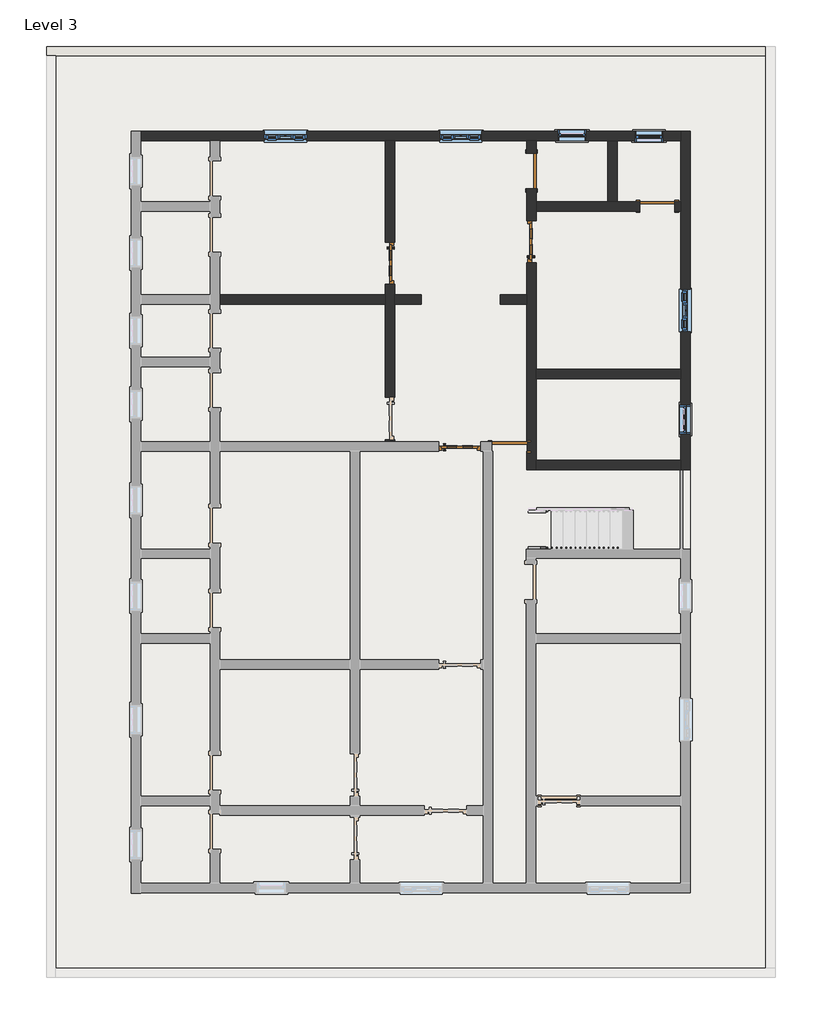
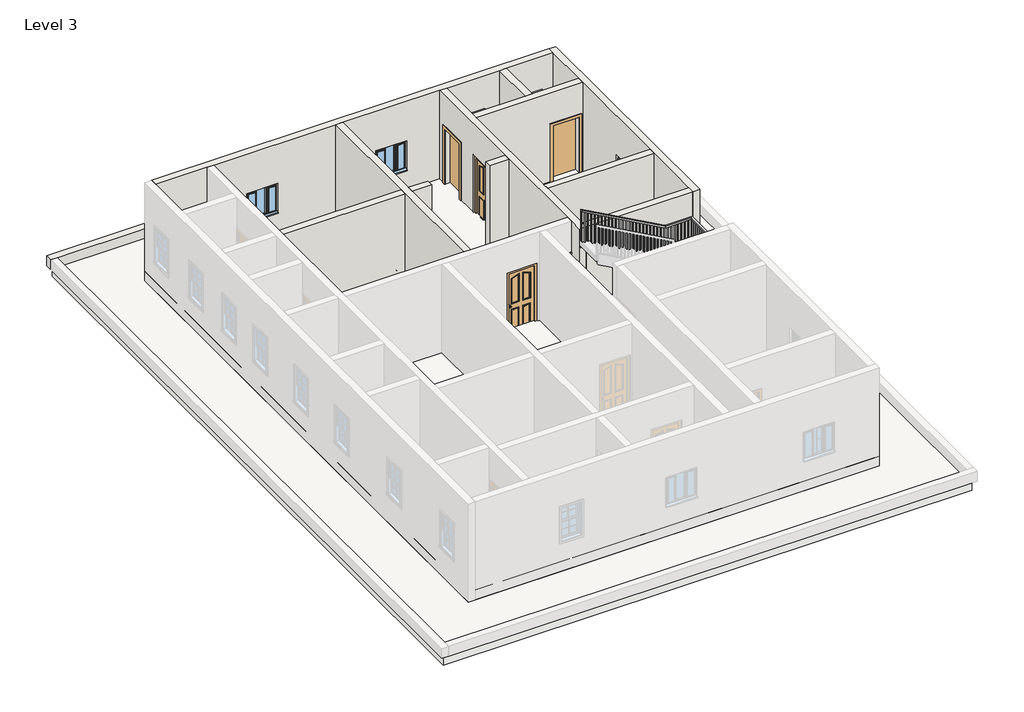
# One storey, part 2 of 3: 11 walls, 6 doors, 6 windows, 2 slabs, 1 railing, 1 roof.
"""IFC4 building model written with IfcOpenShell, lengths in millimetres."""

from ifc_helpers import new_model, si_unit, frame, origin, place, context, project, spatial, polyline, outline, extrude, faceted_brep, transform, mapped, element, save
from components import doors_extsgl_12_910x2110mm_9a09825e, doors_extsgl_12_910x2110mm_ece77ece, door_fadea3f2, window_679d2811, windows_tpl_w_glazing_cross_bars_910x910mm_4aa0f884

model = new_model("IFC4")

# Units and contexts
model_context = context("Model", 3, world=origin())
ifc_project = project(units=[si_unit("LENGTHUNIT", "METRE", prefix="MILLI")], contexts=[model_context])

# Site, building, storey
site = spatial("IfcSite", under=ifc_project)
building = spatial("IfcBuilding", under=site)
storey = spatial("IfcBuildingStorey", under=building, Name="Level 3", Elevation=6096.0)

# Doors
placement = place(None, origin())
doors_extsgl_12_910x2110mm_shape = doors_extsgl_12_910x2110mm_9a09825e(model_context)
element("IfcDoor", 1, ObjectType="Doors_ExtSgl_12 : 910x2110mm", at=placement, inside=storey, context=model_context, shape_type="MappedRepresentation", body=[
    mapped(doors_extsgl_12_910x2110mm_shape, transform((-4887.6876145, 4566.1404944, 6096.0), x_axis=(0.0, -1.0, 0.0), y_axis=(1.0, 0.0, 0.0), z_axis=(0.0, 0.0, 1.0))),
])
element("IfcDoor", 2, ObjectType="Doors_ExtSgl_12 : 910x2110mm", at=placement, inside=storey, context=model_context, shape_type="MappedRepresentation", body=[
    mapped(doors_extsgl_12_910x2110mm_shape, transform((-1839.6876145, 5029.6904944, 6096.0), x_axis=(0.0, 1.0, 0.0), y_axis=(-1.0, 0.0, 0.0), z_axis=(0.0, 0.0, 1.0))),
])
doors_extsgl_12_910x2110mm_2_shape = doors_extsgl_12_910x2110mm_ece77ece(model_context)
element("IfcDoor", 3, ObjectType="Doors_ExtSgl_12 : 910x2110mm", at=placement, inside=storey, context=model_context, shape_type="MappedRepresentation", body=[
    mapped(doors_extsgl_12_910x2110mm_2_shape, transform((-3389.0876145, 603.7404944, 6096.0), x_axis=(1.0, 0.0, 0.0), y_axis=(0.0, 1.0, 0.0), z_axis=(0.0, 0.0, 1.0))),
])
door_shape = door_fadea3f2(model_context)
element("IfcDoor", 4, ObjectType="Single-Flush : 30\" x 80\"", at=placement, inside=storey, context=model_context, shape_type="MappedRepresentation", body=[
    mapped(door_shape, transform((-1839.6876145, 6550.5154944, 6096.0), x_axis=(0.0, -1.0, 0.0), y_axis=(1.0, 0.0, 0.0), z_axis=(0.0, 0.0, 1.0))),
])
element("IfcDoor", 5, ObjectType="Single-Flush : 30\" x 80\"", at=placement, inside=storey, context=model_context, shape_type="MappedRepresentation", body=[
    mapped(door_shape, transform((878.1123855, 5791.6904944, 6096.0), x_axis=(1.0, 0.0, 0.0), y_axis=(0.0, 1.0, 0.0), z_axis=(0.0, 0.0, 1.0))),
])
element("IfcDoor", 6, ObjectType="Single-Flush : 30\" x 80\"", at=placement, inside=storey, context=model_context, shape_type="MappedRepresentation", body=[
    mapped(door_shape, transform((-2309.5876145, 603.7404944, 6096.0), x_axis=(1.0, 0.0, 0.0), y_axis=(0.0, 1.0, 0.0), z_axis=(0.0, 0.0, 1.0))),
])

# Railing
element("IfcRailing", 7, ObjectType="Handrail - Rectangular", at=placement, inside=storey, context=model_context, shape_type="SolidModel", body=[
    faceted_brep([(-1903.1876145, -1555.2595056, 7147.56), (-1903.1876145, -1555.2595056, 7089.4879132), (-1903.1876145, -1606.0595056, 7089.4879132), (-1903.1876145, -1606.0595056, 7147.56), (325.4830625, -1555.2595056, 8382.0), (338.6121628, -1555.2595056, 8331.2), (338.6121628, -1606.0595056, 8331.2), (325.4830625, -1606.0595056, 8382.0), (1322.6123855, -1555.2595056, 8382.0), (1322.6123855, -1555.2595056, 8331.2), (1373.4123855, -1606.0595056, 8331.2), (1373.4123855, -1606.0595056, 8382.0), (1322.6123855, 57.6404944, 8382.0), (1322.6123855, 57.6404944, 8331.2), (1373.4123855, 108.4404944, 8331.2), (1373.4123855, 108.4404944, 8382.0), (573.1131377, 57.6404944, 8382.0), (559.9840375, 57.6404944, 8331.2), (559.9840375, 108.4404944, 8331.2), (573.1131377, 108.4404944, 8382.0), (-1903.1876145, 57.6404944, 9753.6), (-1903.1876145, 108.4404944, 9753.6), (-1903.1876145, 108.4404944, 9695.5279132), (-1903.1876145, 57.6404944, 9695.5279132)], [[[0, 1, 2, 3]], [[1, 0, 4, 5]], [[2, 1, 5, 6]], [[3, 2, 6, 7]], [[0, 3, 7, 4]], [[5, 4, 8, 9]], [[6, 5, 9, 10]], [[7, 6, 10, 11]], [[4, 7, 11, 8]], [[9, 8, 12, 13]], [[10, 9, 13, 14]], [[11, 10, 14, 15]], [[8, 11, 15, 12]], [[13, 12, 16, 17]], [[14, 13, 17, 18]], [[15, 14, 18, 19]], [[12, 15, 19, 16]], [[20, 21, 22, 23]], [[17, 16, 20, 23]], [[18, 17, 23, 22]], [[19, 18, 22, 21]], [[16, 19, 21, 20]]]),
    extrude(outline(polyline([(9633.9768073, -1792.0626145), (9644.5284254, -1811.1126145), (8702.04, -1811.1126145), (8702.04, -1792.0626145), (9633.9768073, -1792.0626145)])), frame((0.0, 73.5154944, 0.0), z_axis=(0.0, 1.0, 0.0), x_axis=(0.0, 0.0, 1.0)), (0.0, 0.0, 1.0), 19.05),
    extrude(outline(polyline([(9577.7015104, -1690.4626145), (9588.2531286, -1709.5126145), (8702.04, -1709.5126145), (8702.04, -1690.4626145), (9577.7015104, -1690.4626145)])), frame((0.0, 73.5154944, 0.0), z_axis=(0.0, 1.0, 0.0), x_axis=(0.0, 0.0, 1.0)), (0.0, 0.0, 1.0), 19.05),
    extrude(outline(polyline([(9521.4262135, -1588.8626145), (9531.9778317, -1607.9126145), (8564.88, -1607.9126145), (8564.88, -1588.8626145), (9521.4262135, -1588.8626145)])), frame((0.0, 73.5154944, 0.0), z_axis=(0.0, 1.0, 0.0), x_axis=(0.0, 0.0, 1.0)), (0.0, 0.0, 1.0), 19.05),
    extrude(outline(polyline([(9465.1509166, -1487.2626145), (9475.7025348, -1506.3126145), (8564.88, -1506.3126145), (8564.88, -1487.2626145), (9465.1509166, -1487.2626145)])), frame((0.0, 73.5154944, 0.0), z_axis=(0.0, 1.0, 0.0), x_axis=(0.0, 0.0, 1.0)), (0.0, 0.0, 1.0), 19.05),
    extrude(outline(polyline([(9408.8756198, -1385.6626145), (9419.4272379, -1404.7126145), (8427.72, -1404.7126145), (8427.72, -1385.6626145), (9408.8756198, -1385.6626145)])), frame((0.0, 73.5154944, 0.0), z_axis=(0.0, 1.0, 0.0), x_axis=(0.0, 0.0, 1.0)), (0.0, 0.0, 1.0), 19.05),
    extrude(outline(polyline([(9352.6003229, -1284.0626145), (9363.151941, -1303.1126145), (8427.72, -1303.1126145), (8427.72, -1284.0626145), (9352.6003229, -1284.0626145)])), frame((0.0, 73.5154944, 0.0), z_axis=(0.0, 1.0, 0.0), x_axis=(0.0, 0.0, 1.0)), (0.0, 0.0, 1.0), 19.05),
    extrude(outline(polyline([(9296.325026, -1182.4626145), (9306.8766442, -1201.5126145), (8427.72, -1201.5126145), (8427.72, -1182.4626145), (9296.325026, -1182.4626145)])), frame((0.0, 73.5154944, 0.0), z_axis=(0.0, 1.0, 0.0), x_axis=(0.0, 0.0, 1.0)), (0.0, 0.0, 1.0), 19.05),
    extrude(outline(polyline([(9240.0497291, -1080.8626145), (9250.6013473, -1099.9126145), (8290.56, -1099.9126145), (8290.56, -1080.8626145), (9240.0497291, -1080.8626145)])), frame((0.0, 73.5154944, 0.0), z_axis=(0.0, 1.0, 0.0), x_axis=(0.0, 0.0, 1.0)), (0.0, 0.0, 1.0), 19.05),
    extrude(outline(polyline([(9183.7744322, -979.2626145), (9194.3260504, -998.3126145), (8290.56, -998.3126145), (8290.56, -979.2626145), (9183.7744322, -979.2626145)])), frame((0.0, 73.5154944, 0.0), z_axis=(0.0, 1.0, 0.0), x_axis=(0.0, 0.0, 1.0)), (0.0, 0.0, 1.0), 19.05),
    extrude(outline(polyline([(9127.4991354, -877.6626145), (9138.0507535, -896.7126145), (8153.4, -896.7126145), (8153.4, -877.6626145), (9127.4991354, -877.6626145)])), frame((0.0, 73.5154944, 0.0), z_axis=(0.0, 1.0, 0.0), x_axis=(0.0, 0.0, 1.0)), (0.0, 0.0, 1.0), 19.05),
    extrude(outline(polyline([(9071.2238385, -776.0626145), (9081.7754566, -795.1126145), (8153.4, -795.1126145), (8153.4, -776.0626145), (9071.2238385, -776.0626145)])), frame((0.0, 73.5154944, 0.0), z_axis=(0.0, 1.0, 0.0), x_axis=(0.0, 0.0, 1.0)), (0.0, 0.0, 1.0), 19.05),
    extrude(outline(polyline([(9014.9485416, -674.4626145), (9025.5001598, -693.5126145), (8153.4, -693.5126145), (8153.4, -674.4626145), (9014.9485416, -674.4626145)])), frame((0.0, 73.5154944, 0.0), z_axis=(0.0, 1.0, 0.0), x_axis=(0.0, 0.0, 1.0)), (0.0, 0.0, 1.0), 19.05),
    extrude(outline(polyline([(8958.6732447, -572.8626145), (8969.2248629, -591.9126145), (8016.24, -591.9126145), (8016.24, -572.8626145), (8958.6732447, -572.8626145)])), frame((0.0, 73.5154944, 0.0), z_axis=(0.0, 1.0, 0.0), x_axis=(0.0, 0.0, 1.0)), (0.0, 0.0, 1.0), 19.05),
    extrude(outline(polyline([(8902.3979478, -471.2626145), (8912.949566, -490.3126145), (8016.24, -490.3126145), (8016.24, -471.2626145), (8902.3979478, -471.2626145)])), frame((0.0, 73.5154944, 0.0), z_axis=(0.0, 1.0, 0.0), x_axis=(0.0, 0.0, 1.0)), (0.0, 0.0, 1.0), 19.05),
    extrude(outline(polyline([(8846.1226509, -369.6626145), (8856.6742691, -388.7126145), (7879.08, -388.7126145), (7879.08, -369.6626145), (8846.1226509, -369.6626145)])), frame((0.0, 73.5154944, 0.0), z_axis=(0.0, 1.0, 0.0), x_axis=(0.0, 0.0, 1.0)), (0.0, 0.0, 1.0), 19.05),
    extrude(outline(polyline([(8789.8473541, -268.0626145), (8800.3989722, -287.1126145), (7879.08, -287.1126145), (7879.08, -268.0626145), (8789.8473541, -268.0626145)])), frame((0.0, 73.5154944, 0.0), z_axis=(0.0, 1.0, 0.0), x_axis=(0.0, 0.0, 1.0)), (0.0, 0.0, 1.0), 19.05),
    extrude(outline(polyline([(8733.5720572, -166.4626145), (8744.1236754, -185.5126145), (7879.08, -185.5126145), (7879.08, -166.4626145), (8733.5720572, -166.4626145)])), frame((0.0, 73.5154944, 0.0), z_axis=(0.0, 1.0, 0.0), x_axis=(0.0, 0.0, 1.0)), (0.0, 0.0, 1.0), 19.05),
    extrude(outline(polyline([(8677.2967603, -64.8626145), (8687.8483785, -83.9126145), (7741.92, -83.9126145), (7741.92, -64.8626145), (8677.2967603, -64.8626145)])), frame((0.0, 73.5154944, 0.0), z_axis=(0.0, 1.0, 0.0), x_axis=(0.0, 0.0, 1.0)), (0.0, 0.0, 1.0), 19.05),
    extrude(outline(polyline([(8621.0214634, 36.7373855), (8631.5730816, 17.6873855), (7741.92, 17.6873855), (7741.92, 36.7373855), (8621.0214634, 36.7373855)])), frame((0.0, 73.5154944, 0.0), z_axis=(0.0, 1.0, 0.0), x_axis=(0.0, 0.0, 1.0)), (0.0, 0.0, 1.0), 19.05),
    extrude(outline(polyline([(8564.7461665, 138.3373855), (8575.2977847, 119.2873855), (7604.76, 119.2873855), (7604.76, 138.3373855), (8564.7461665, 138.3373855)])), frame((0.0, 73.5154944, 0.0), z_axis=(0.0, 1.0, 0.0), x_axis=(0.0, 0.0, 1.0)), (0.0, 0.0, 1.0), 19.05),
    extrude(outline(polyline([(8508.4708697, 239.9373855), (8519.0224878, 220.8873855), (7604.76, 220.8873855), (7604.76, 239.9373855), (8508.4708697, 239.9373855)])), frame((0.0, 73.5154944, 0.0), z_axis=(0.0, 1.0, 0.0), x_axis=(0.0, 0.0, 1.0)), (0.0, 0.0, 1.0), 19.05),
    extrude(outline(polyline([(8452.1955728, 341.5373855), (8462.7471909, 322.4873855), (7467.6, 322.4873855), (7467.6, 341.5373855), (8452.1955728, 341.5373855)])), frame((0.0, 73.5154944, 0.0), z_axis=(0.0, 1.0, 0.0), x_axis=(0.0, 0.0, 1.0)), (0.0, 0.0, 1.0), 19.05),
    extrude(outline(polyline([(8395.9202759, 443.1373855), (8406.4718941, 424.0873855), (7467.6, 424.0873855), (7467.6, 443.1373855), (8395.9202759, 443.1373855)])), frame((0.0, 73.5154944, 0.0), z_axis=(0.0, 1.0, 0.0), x_axis=(0.0, 0.0, 1.0)), (0.0, 0.0, 1.0), 19.05),
    extrude(outline(polyline([(8339.644979, 544.7373855), (8350.1965972, 525.6873855), (7467.6, 525.6873855), (7467.6, 544.7373855), (8339.644979, 544.7373855)])), frame((0.0, 73.5154944, 0.0), z_axis=(0.0, 1.0, 0.0), x_axis=(0.0, 0.0, 1.0)), (0.0, 0.0, 1.0), 19.05),
    extrude(outline(polyline([(646.3373855, 92.5654944), (646.3373855, 73.5154944), (627.2873855, 73.5154944), (627.2873855, 92.5654944), (646.3373855, 92.5654944)])), frame((0.0, 0.0, 7467.6), z_axis=(0.0, 0.0, 1.0), x_axis=(1.0, 0.0, 0.0)), (0.0, 0.0, 1.0), 863.6),
    extrude(outline(polyline([(747.9373855, 92.5654944), (747.9373855, 73.5154944), (728.8873855, 73.5154944), (728.8873855, 92.5654944), (747.9373855, 92.5654944)])), frame((0.0, 0.0, 7467.6), z_axis=(0.0, 0.0, 1.0), x_axis=(1.0, 0.0, 0.0)), (0.0, 0.0, 1.0), 863.6),
    extrude(outline(polyline([(849.5373855, 92.5654944), (849.5373855, 73.5154944), (830.4873855, 73.5154944), (830.4873855, 92.5654944), (849.5373855, 92.5654944)])), frame((0.0, 0.0, 7467.6), z_axis=(0.0, 0.0, 1.0), x_axis=(1.0, 0.0, 0.0)), (0.0, 0.0, 1.0), 863.6),
    extrude(outline(polyline([(951.1373855, 92.5654944), (951.1373855, 73.5154944), (932.0873855, 73.5154944), (932.0873855, 92.5654944), (951.1373855, 92.5654944)])), frame((0.0, 0.0, 7467.6), z_axis=(0.0, 0.0, 1.0), x_axis=(1.0, 0.0, 0.0)), (0.0, 0.0, 1.0), 863.6),
    extrude(outline(polyline([(1052.7373855, 92.5654944), (1052.7373855, 73.5154944), (1033.6873855, 73.5154944), (1033.6873855, 92.5654944), (1052.7373855, 92.5654944)])), frame((0.0, 0.0, 7467.6), z_axis=(0.0, 0.0, 1.0), x_axis=(1.0, 0.0, 0.0)), (0.0, 0.0, 1.0), 863.6),
    extrude(outline(polyline([(1154.3373855, 92.5654944), (1154.3373855, 73.5154944), (1135.2873855, 73.5154944), (1135.2873855, 92.5654944), (1154.3373855, 92.5654944)])), frame((0.0, 0.0, 7467.6), z_axis=(0.0, 0.0, 1.0), x_axis=(1.0, 0.0, 0.0)), (0.0, 0.0, 1.0), 863.6),
    extrude(outline(polyline([(1255.9373855, 92.5654944), (1255.9373855, 73.5154944), (1236.8873855, 73.5154944), (1236.8873855, 92.5654944), (1255.9373855, 92.5654944)])), frame((0.0, 0.0, 7467.6), z_axis=(0.0, 0.0, 1.0), x_axis=(1.0, 0.0, 0.0)), (0.0, 0.0, 1.0), 863.6),
    extrude(outline(polyline([(1357.5373855, 35.4154944), (1338.4873855, 35.4154944), (1338.4873855, 54.4654944), (1357.5373855, 54.4654944), (1357.5373855, 35.4154944)])), frame((0.0, 0.0, 7467.6), z_axis=(0.0, 0.0, 1.0), x_axis=(1.0, 0.0, 0.0)), (0.0, 0.0, 1.0), 863.6),
    extrude(outline(polyline([(1357.5373855, -66.1845056), (1338.4873855, -66.1845056), (1338.4873855, -47.1345056), (1357.5373855, -47.1345056), (1357.5373855, -66.1845056)])), frame((0.0, 0.0, 7467.6), z_axis=(0.0, 0.0, 1.0), x_axis=(1.0, 0.0, 0.0)), (0.0, 0.0, 1.0), 863.6),
    extrude(outline(polyline([(1357.5373855, -167.7845056), (1338.4873855, -167.7845056), (1338.4873855, -148.7345056), (1357.5373855, -148.7345056), (1357.5373855, -167.7845056)])), frame((0.0, 0.0, 7467.6), z_axis=(0.0, 0.0, 1.0), x_axis=(1.0, 0.0, 0.0)), (0.0, 0.0, 1.0), 863.6),
    extrude(outline(polyline([(1357.5373855, -269.3845056), (1338.4873855, -269.3845056), (1338.4873855, -250.3345056), (1357.5373855, -250.3345056), (1357.5373855, -269.3845056)])), frame((0.0, 0.0, 7467.6), z_axis=(0.0, 0.0, 1.0), x_axis=(1.0, 0.0, 0.0)), (0.0, 0.0, 1.0), 863.6),
    extrude(outline(polyline([(1357.5373855, -370.9845056), (1338.4873855, -370.9845056), (1338.4873855, -351.9345056), (1357.5373855, -351.9345056), (1357.5373855, -370.9845056)])), frame((0.0, 0.0, 7467.6), z_axis=(0.0, 0.0, 1.0), x_axis=(1.0, 0.0, 0.0)), (0.0, 0.0, 1.0), 863.6),
    extrude(outline(polyline([(1357.5373855, -472.5845056), (1338.4873855, -472.5845056), (1338.4873855, -453.5345056), (1357.5373855, -453.5345056), (1357.5373855, -472.5845056)])), frame((0.0, 0.0, 7467.6), z_axis=(0.0, 0.0, 1.0), x_axis=(1.0, 0.0, 0.0)), (0.0, 0.0, 1.0), 863.6),
    extrude(outline(polyline([(1357.5373855, -574.1845056), (1338.4873855, -574.1845056), (1338.4873855, -555.1345056), (1357.5373855, -555.1345056), (1357.5373855, -574.1845056)])), frame((0.0, 0.0, 7467.6), z_axis=(0.0, 0.0, 1.0), x_axis=(1.0, 0.0, 0.0)), (0.0, 0.0, 1.0), 863.6),
    extrude(outline(polyline([(1357.5373855, -675.7845056), (1338.4873855, -675.7845056), (1338.4873855, -656.7345056), (1357.5373855, -656.7345056), (1357.5373855, -675.7845056)])), frame((0.0, 0.0, 7467.6), z_axis=(0.0, 0.0, 1.0), x_axis=(1.0, 0.0, 0.0)), (0.0, 0.0, 1.0), 863.6),
    extrude(outline(polyline([(1357.5373855, -777.3845056), (1338.4873855, -777.3845056), (1338.4873855, -758.3345056), (1357.5373855, -758.3345056), (1357.5373855, -777.3845056)])), frame((0.0, 0.0, 7467.6), z_axis=(0.0, 0.0, 1.0), x_axis=(1.0, 0.0, 0.0)), (0.0, 0.0, 1.0), 863.6),
    extrude(outline(polyline([(1357.5373855, -878.9845056), (1338.4873855, -878.9845056), (1338.4873855, -859.9345056), (1357.5373855, -859.9345056), (1357.5373855, -878.9845056)])), frame((0.0, 0.0, 7467.6), z_axis=(0.0, 0.0, 1.0), x_axis=(1.0, 0.0, 0.0)), (0.0, 0.0, 1.0), 863.6),
    extrude(outline(polyline([(1357.5373855, -980.5845056), (1338.4873855, -980.5845056), (1338.4873855, -961.5345056), (1357.5373855, -961.5345056), (1357.5373855, -980.5845056)])), frame((0.0, 0.0, 7467.6), z_axis=(0.0, 0.0, 1.0), x_axis=(1.0, 0.0, 0.0)), (0.0, 0.0, 1.0), 863.6),
    extrude(outline(polyline([(1357.5373855, -1082.1845056), (1338.4873855, -1082.1845056), (1338.4873855, -1063.1345056), (1357.5373855, -1063.1345056), (1357.5373855, -1082.1845056)])), frame((0.0, 0.0, 7467.6), z_axis=(0.0, 0.0, 1.0), x_axis=(1.0, 0.0, 0.0)), (0.0, 0.0, 1.0), 863.6),
    extrude(outline(polyline([(1357.5373855, -1183.7845056), (1338.4873855, -1183.7845056), (1338.4873855, -1164.7345056), (1357.5373855, -1164.7345056), (1357.5373855, -1183.7845056)])), frame((0.0, 0.0, 7467.6), z_axis=(0.0, 0.0, 1.0), x_axis=(1.0, 0.0, 0.0)), (0.0, 0.0, 1.0), 863.6),
    extrude(outline(polyline([(1357.5373855, -1285.3845056), (1338.4873855, -1285.3845056), (1338.4873855, -1266.3345056), (1357.5373855, -1266.3345056), (1357.5373855, -1285.3845056)])), frame((0.0, 0.0, 7467.6), z_axis=(0.0, 0.0, 1.0), x_axis=(1.0, 0.0, 0.0)), (0.0, 0.0, 1.0), 863.6),
    extrude(outline(polyline([(1357.5373855, -1386.9845056), (1338.4873855, -1386.9845056), (1338.4873855, -1367.9345056), (1357.5373855, -1367.9345056), (1357.5373855, -1386.9845056)])), frame((0.0, 0.0, 7467.6), z_axis=(0.0, 0.0, 1.0), x_axis=(1.0, 0.0, 0.0)), (0.0, 0.0, 1.0), 863.6),
    extrude(outline(polyline([(1357.5373855, -1488.5845056), (1338.4873855, -1488.5845056), (1338.4873855, -1469.5345056), (1357.5373855, -1469.5345056), (1357.5373855, -1488.5845056)])), frame((0.0, 0.0, 7467.6), z_axis=(0.0, 0.0, 1.0), x_axis=(1.0, 0.0, 0.0)), (0.0, 0.0, 1.0), 863.6),
    extrude(outline(polyline([(1236.8873855, -1590.1845056), (1236.8873855, -1571.1345056), (1255.9373855, -1571.1345056), (1255.9373855, -1590.1845056), (1236.8873855, -1590.1845056)])), frame((0.0, 0.0, 7467.6), z_axis=(0.0, 0.0, 1.0), x_axis=(1.0, 0.0, 0.0)), (0.0, 0.0, 1.0), 863.6),
    extrude(outline(polyline([(1135.2873855, -1590.1845056), (1135.2873855, -1571.1345056), (1154.3373855, -1571.1345056), (1154.3373855, -1590.1845056), (1135.2873855, -1590.1845056)])), frame((0.0, 0.0, 7467.6), z_axis=(0.0, 0.0, 1.0), x_axis=(1.0, 0.0, 0.0)), (0.0, 0.0, 1.0), 863.6),
    extrude(outline(polyline([(1033.6873855, -1590.1845056), (1033.6873855, -1571.1345056), (1052.7373855, -1571.1345056), (1052.7373855, -1590.1845056), (1033.6873855, -1590.1845056)])), frame((0.0, 0.0, 7467.6), z_axis=(0.0, 0.0, 1.0), x_axis=(1.0, 0.0, 0.0)), (0.0, 0.0, 1.0), 863.6),
    extrude(outline(polyline([(932.0873855, -1590.1845056), (932.0873855, -1571.1345056), (951.1373855, -1571.1345056), (951.1373855, -1590.1845056), (932.0873855, -1590.1845056)])), frame((0.0, 0.0, 7467.6), z_axis=(0.0, 0.0, 1.0), x_axis=(1.0, 0.0, 0.0)), (0.0, 0.0, 1.0), 863.6),
    extrude(outline(polyline([(830.4873855, -1590.1845056), (830.4873855, -1571.1345056), (849.5373855, -1571.1345056), (849.5373855, -1590.1845056), (830.4873855, -1590.1845056)])), frame((0.0, 0.0, 7467.6), z_axis=(0.0, 0.0, 1.0), x_axis=(1.0, 0.0, 0.0)), (0.0, 0.0, 1.0), 863.6),
    extrude(outline(polyline([(728.8873855, -1590.1845056), (728.8873855, -1571.1345056), (747.9373855, -1571.1345056), (747.9373855, -1590.1845056), (728.8873855, -1590.1845056)])), frame((0.0, 0.0, 7467.6), z_axis=(0.0, 0.0, 1.0), x_axis=(1.0, 0.0, 0.0)), (0.0, 0.0, 1.0), 863.6),
    extrude(outline(polyline([(627.2873855, -1590.1845056), (627.2873855, -1571.1345056), (646.3373855, -1571.1345056), (646.3373855, -1590.1845056), (627.2873855, -1590.1845056)])), frame((0.0, 0.0, 7467.6), z_axis=(0.0, 0.0, 1.0), x_axis=(1.0, 0.0, 0.0)), (0.0, 0.0, 1.0), 863.6),
    extrude(outline(polyline([(525.6873855, -1590.1845056), (525.6873855, -1571.1345056), (544.7373855, -1571.1345056), (544.7373855, -1590.1845056), (525.6873855, -1590.1845056)])), frame((0.0, 0.0, 7467.6), z_axis=(0.0, 0.0, 1.0), x_axis=(1.0, 0.0, 0.0)), (0.0, 0.0, 1.0), 863.6),
    extrude(outline(polyline([(424.0873855, -1590.1845056), (424.0873855, -1571.1345056), (443.1373855, -1571.1345056), (443.1373855, -1590.1845056), (424.0873855, -1590.1845056)])), frame((0.0, 0.0, 7467.6), z_axis=(0.0, 0.0, 1.0), x_axis=(1.0, 0.0, 0.0)), (0.0, 0.0, 1.0), 863.6),
    extrude(outline(polyline([(322.4873855, -1590.1845056), (322.4873855, -1571.1345056), (341.5373855, -1571.1345056), (341.5373855, -1590.1845056), (322.4873855, -1590.1845056)])), frame((0.0, 0.0, 7467.6), z_axis=(0.0, 0.0, 1.0), x_axis=(1.0, 0.0, 0.0)), (0.0, 0.0, 1.0), 863.6),
    extrude(outline(polyline([(8276.5449568, 239.9373855), (8265.9933387, 220.8873855), (7330.44, 220.8873855), (7330.44, 239.9373855), (8276.5449568, 239.9373855)])), frame((0.0, -1590.1845056, 0.0), z_axis=(0.0, 1.0, 0.0), x_axis=(0.0, 0.0, 1.0)), (0.0, 0.0, 1.0), 19.05),
    extrude(outline(polyline([(8220.2696599, 138.3373855), (8209.7180418, 119.2873855), (7330.44, 119.2873855), (7330.44, 138.3373855), (8220.2696599, 138.3373855)])), frame((0.0, -1590.1845056, 0.0), z_axis=(0.0, 1.0, 0.0), x_axis=(0.0, 0.0, 1.0)), (0.0, 0.0, 1.0), 19.05),
    extrude(outline(polyline([(8163.9943631, 36.7373855), (8153.4427449, 17.6873855), (7193.28, 17.6873855), (7193.28, 36.7373855), (8163.9943631, 36.7373855)])), frame((0.0, -1590.1845056, 0.0), z_axis=(0.0, 1.0, 0.0), x_axis=(0.0, 0.0, 1.0)), (0.0, 0.0, 1.0), 19.05),
    extrude(outline(polyline([(8107.7190662, -64.8626145), (8097.167448, -83.9126145), (7193.28, -83.9126145), (7193.28, -64.8626145), (8107.7190662, -64.8626145)])), frame((0.0, -1590.1845056, 0.0), z_axis=(0.0, 1.0, 0.0), x_axis=(0.0, 0.0, 1.0)), (0.0, 0.0, 1.0), 19.05),
    extrude(outline(polyline([(8051.4437693, -166.4626145), (8040.8921511, -185.5126145), (7056.12, -185.5126145), (7056.12, -166.4626145), (8051.4437693, -166.4626145)])), frame((0.0, -1590.1845056, 0.0), z_axis=(0.0, 1.0, 0.0), x_axis=(0.0, 0.0, 1.0)), (0.0, 0.0, 1.0), 19.05),
    extrude(outline(polyline([(7995.1684724, -268.0626145), (7984.6168543, -287.1126145), (7056.12, -287.1126145), (7056.12, -268.0626145), (7995.1684724, -268.0626145)])), frame((0.0, -1590.1845056, 0.0), z_axis=(0.0, 1.0, 0.0), x_axis=(0.0, 0.0, 1.0)), (0.0, 0.0, 1.0), 19.05),
    extrude(outline(polyline([(7938.8931755, -369.6626145), (7928.3415574, -388.7126145), (7056.12, -388.7126145), (7056.12, -369.6626145), (7938.8931755, -369.6626145)])), frame((0.0, -1590.1845056, 0.0), z_axis=(0.0, 1.0, 0.0), x_axis=(0.0, 0.0, 1.0)), (0.0, 0.0, 1.0), 19.05),
    extrude(outline(polyline([(7882.6178787, -471.2626145), (7872.0662605, -490.3126145), (6918.96, -490.3126145), (6918.96, -471.2626145), (7882.6178787, -471.2626145)])), frame((0.0, -1590.1845056, 0.0), z_axis=(0.0, 1.0, 0.0), x_axis=(0.0, 0.0, 1.0)), (0.0, 0.0, 1.0), 19.05),
    extrude(outline(polyline([(7826.3425818, -572.8626145), (7815.7909636, -591.9126145), (6918.96, -591.9126145), (6918.96, -572.8626145), (7826.3425818, -572.8626145)])), frame((0.0, -1590.1845056, 0.0), z_axis=(0.0, 1.0, 0.0), x_axis=(0.0, 0.0, 1.0)), (0.0, 0.0, 1.0), 19.05),
    extrude(outline(polyline([(7770.0672849, -674.4626145), (7759.5156667, -693.5126145), (6781.8, -693.5126145), (6781.8, -674.4626145), (7770.0672849, -674.4626145)])), frame((0.0, -1590.1845056, 0.0), z_axis=(0.0, 1.0, 0.0), x_axis=(0.0, 0.0, 1.0)), (0.0, 0.0, 1.0), 19.05),
    extrude(outline(polyline([(7713.791988, -776.0626145), (7703.2403699, -795.1126145), (6781.8, -795.1126145), (6781.8, -776.0626145), (7713.791988, -776.0626145)])), frame((0.0, -1590.1845056, 0.0), z_axis=(0.0, 1.0, 0.0), x_axis=(0.0, 0.0, 1.0)), (0.0, 0.0, 1.0), 19.05),
    extrude(outline(polyline([(7657.5166911, -877.6626145), (7646.965073, -896.7126145), (6781.8, -896.7126145), (6781.8, -877.6626145), (7657.5166911, -877.6626145)])), frame((0.0, -1590.1845056, 0.0), z_axis=(0.0, 1.0, 0.0), x_axis=(0.0, 0.0, 1.0)), (0.0, 0.0, 1.0), 19.05),
    extrude(outline(polyline([(7601.2413943, -979.2626145), (7590.6897761, -998.3126145), (6644.64, -998.3126145), (6644.64, -979.2626145), (7601.2413943, -979.2626145)])), frame((0.0, -1590.1845056, 0.0), z_axis=(0.0, 1.0, 0.0), x_axis=(0.0, 0.0, 1.0)), (0.0, 0.0, 1.0), 19.05),
    extrude(outline(polyline([(7544.9660974, -1080.8626145), (7534.4144792, -1099.9126145), (6644.64, -1099.9126145), (6644.64, -1080.8626145), (7544.9660974, -1080.8626145)])), frame((0.0, -1590.1845056, 0.0), z_axis=(0.0, 1.0, 0.0), x_axis=(0.0, 0.0, 1.0)), (0.0, 0.0, 1.0), 19.05),
    extrude(outline(polyline([(7488.6908005, -1182.4626145), (7478.1391823, -1201.5126145), (6507.48, -1201.5126145), (6507.48, -1182.4626145), (7488.6908005, -1182.4626145)])), frame((0.0, -1590.1845056, 0.0), z_axis=(0.0, 1.0, 0.0), x_axis=(0.0, 0.0, 1.0)), (0.0, 0.0, 1.0), 19.05),
    extrude(outline(polyline([(7432.4155036, -1284.0626145), (7421.8638855, -1303.1126145), (6507.48, -1303.1126145), (6507.48, -1284.0626145), (7432.4155036, -1284.0626145)])), frame((0.0, -1590.1845056, 0.0), z_axis=(0.0, 1.0, 0.0), x_axis=(0.0, 0.0, 1.0)), (0.0, 0.0, 1.0), 19.05),
    extrude(outline(polyline([(7376.1402067, -1385.6626145), (7365.5885886, -1404.7126145), (6507.48, -1404.7126145), (6507.48, -1385.6626145), (7376.1402067, -1385.6626145)])), frame((0.0, -1590.1845056, 0.0), z_axis=(0.0, 1.0, 0.0), x_axis=(0.0, 0.0, 1.0)), (0.0, 0.0, 1.0), 19.05),
    extrude(outline(polyline([(7319.8649099, -1487.2626145), (7309.3132917, -1506.3126145), (6370.32, -1506.3126145), (6370.32, -1487.2626145), (7319.8649099, -1487.2626145)])), frame((0.0, -1590.1845056, 0.0), z_axis=(0.0, 1.0, 0.0), x_axis=(0.0, 0.0, 1.0)), (0.0, 0.0, 1.0), 19.05),
    extrude(outline(polyline([(7263.589613, -1588.8626145), (7253.0379948, -1607.9126145), (6370.32, -1607.9126145), (6370.32, -1588.8626145), (7263.589613, -1588.8626145)])), frame((0.0, -1590.1845056, 0.0), z_axis=(0.0, 1.0, 0.0), x_axis=(0.0, 0.0, 1.0)), (0.0, 0.0, 1.0), 19.05),
    extrude(outline(polyline([(7207.3143161, -1690.4626145), (7196.7626979, -1709.5126145), (6233.16, -1709.5126145), (6233.16, -1690.4626145), (7207.3143161, -1690.4626145)])), frame((0.0, -1590.1845056, 0.0), z_axis=(0.0, 1.0, 0.0), x_axis=(0.0, 0.0, 1.0)), (0.0, 0.0, 1.0), 19.05),
    extrude(outline(polyline([(7151.0390192, -1792.0626145), (7140.487401, -1811.1126145), (6233.16, -1811.1126145), (6233.16, -1792.0626145), (7151.0390192, -1792.0626145)])), frame((0.0, -1590.1845056, 0.0), z_axis=(0.0, 1.0, 0.0), x_axis=(0.0, 0.0, 1.0)), (0.0, 0.0, 1.0), 19.05),
    extrude(outline(polyline([(1357.5373855, 73.5154944), (1338.4873855, 73.5154944), (1338.4873855, 92.5654944), (1357.5373855, 92.5654944), (1357.5373855, 73.5154944)])), frame((0.0, 0.0, 7467.6), z_axis=(0.0, 0.0, 1.0), x_axis=(1.0, 0.0, 0.0)), (0.0, 0.0, 1.0), 863.6),
    extrude(outline(polyline([(1338.4873855, -1590.1845056), (1338.4873855, -1571.1345056), (1357.5373855, -1571.1345056), (1357.5373855, -1590.1845056), (1338.4873855, -1590.1845056)])), frame((0.0, 0.0, 7467.6), z_axis=(0.0, 0.0, 1.0), x_axis=(1.0, 0.0, 0.0)), (0.0, 0.0, 1.0), 863.6),
    extrude(outline(polyline([(9684.9762951, -1884.1376145), (9695.5279132, -1903.1876145), (8702.04, -1903.1876145), (8702.04, -1884.1376145), (9684.9762951, -1884.1376145)])), frame((0.0, 73.5154944, 0.0), z_axis=(0.0, 1.0, 0.0), x_axis=(0.0, 0.0, 1.0)), (0.0, 0.0, 1.0), 19.05),
    extrude(outline(polyline([(7100.0395314, -1884.1376145), (7089.4879132, -1903.1876145), (6233.16, -1903.1876145), (6233.16, -1884.1376145), (7100.0395314, -1884.1376145)])), frame((0.0, -1590.1845056, 0.0), z_axis=(0.0, 1.0, 0.0), x_axis=(0.0, 0.0, 1.0)), (0.0, 0.0, 1.0), 19.05),
])

# Roof
element("IfcRoof", 8, ObjectType="Generic - 12\"", at=placement, inside=storey, context=model_context, shape_type="SweptSolid", body=[
    extrude(outline(polyline([(-10475.6876145, 7410.9404944), (1589.3123855, 7410.9404944), (1589.3123855, -9022.8595056), (-10475.6876145, -9022.8595056), (-10475.6876145, 7410.9404944)])), frame((0.0, 0.0, 6096.0), z_axis=(0.0, 0.0, 1.0), x_axis=(1.0, 0.0, 0.0)), (0.0, 0.0, 1.0), 304.8),
])

# Slabs
element("IfcSlab", 9, ObjectType="Generic - 12\"", at=placement, inside=storey, context=model_context, shape_type="SweptSolid", body=[
    extrude(outline(polyline([(1589.3123855, 7410.9404944), (1589.3123855, -9022.8595056), (-10475.6876145, -9022.8595056), (-10475.6876145, 7410.9404944), (1589.3123855, 7410.9404944)])), frame((0.0, 0.0, 5791.2), z_axis=(0.0, 0.0, 1.0), x_axis=(1.0, 0.0, 0.0)), (0.0, 0.0, 1.0), 304.8),
])
element("IfcSlab", 10, ObjectType="Generic - 12\"", at=placement, inside=storey, context=model_context, shape_type="SweptSolid", body=[
    extrude(outline(polyline([(3316.5123855, 9138.1404944), (3316.5123855, -10750.0595056), (-12202.8876145, -10750.0595056), (-12202.8876145, 9138.1404944), (3316.5123855, 9138.1404944)])), frame((0.0, 0.0, 5791.2), z_axis=(0.0, 0.0, 1.0), x_axis=(1.0, 0.0, 0.0)), (0.0, 0.0, 1.0), 304.8),
])

# Walls
element("IfcWall", 11, ObjectType="4.5\"", at=placement, inside=storey, context=model_context, shape_type="Brep", body=[
    faceted_brep([(-4989.2876145, 758.3404944, 8206.0), (-4989.2876145, 758.3404944, 6096.0), (-4989.2876145, 705.3404944, 6096.0), (-4989.2876145, 705.3404944, 9144.0), (-4989.2876145, 3677.1404944, 9144.0), (-4989.2876145, 3880.3404944, 9144.0), (-4989.2876145, 7207.7404944, 9144.0), (-4989.2876145, 7207.7404944, 6096.0), (-4989.2876145, 5021.1404944, 6096.0), (-4989.2876145, 5021.1404944, 8206.0), (-4989.2876145, 4111.1404944, 8206.0), (-4989.2876145, 4111.1404944, 6096.0), (-4989.2876145, 3880.3404944, 6096.0), (-4989.2876145, 3677.1404944, 6096.0), (-4989.2876145, 1668.3404944, 6096.0), (-4989.2876145, 1668.3404944, 8206.0), (-4786.0876145, 705.3404944, 6096.0), (-4786.0876145, 758.3404944, 6096.0), (-4786.0876145, 758.3404944, 8206.0), (-4786.0876145, 1668.3404944, 8206.0), (-4786.0876145, 1668.3404944, 6096.0), (-4786.0876145, 3677.1404944, 6096.0), (-4786.0876145, 3880.3404944, 6096.0), (-4786.0876145, 4111.1404944, 6096.0), (-4786.0876145, 4111.1404944, 8206.0), (-4786.0876145, 5021.1404944, 8206.0), (-4786.0876145, 5021.1404944, 6096.0), (-4786.0876145, 7207.7404944, 6096.0), (-4786.0876145, 7207.7404944, 9144.0), (-4786.0876145, 3880.3404944, 9144.0), (-4786.0876145, 3677.1404944, 9144.0), (-4786.0876145, 705.3404944, 9144.0)], [[[0, 1, 2, 3, 4, 5, 6, 7, 8, 9, 10, 11, 12, 13, 14, 15]], [[16, 17, 18, 19, 20, 21, 22, 23, 24, 25, 26, 27, 28, 29, 30, 31]], [[8, 7, 27, 26]], [[2, 1, 17, 16]], [[14, 13, 12, 11, 23, 22, 21, 20]], [[6, 5, 4, 3, 31, 30, 29, 28]], [[7, 6, 28, 27]], [[3, 2, 16, 31]], [[26, 25, 9, 8]], [[24, 23, 11, 10]], [[25, 24, 10, 9]], [[20, 19, 15, 14]], [[18, 17, 1, 0]], [[19, 18, 0, 15]]]),
])
element("IfcWall", 12, ObjectType="4.5\"", at=placement, inside=storey, context=model_context, shape_type="SweptSolid", body=[
    extrude(outline(polyline([(-4214.5876145, 3880.3404944), (-4214.5876145, 3677.1404944), (-4786.0876145, 3677.1404944), (-4786.0876145, 3880.3404944), (-4214.5876145, 3880.3404944)])), frame((0.0, 0.0, 6096.0), z_axis=(0.0, 0.0, 1.0), x_axis=(1.0, 0.0, 0.0)), (0.0, 0.0, 1.0), 3048.0),
    extrude(outline(polyline([(-8570.6876145, 3677.1404944), (-8570.6876145, 3880.3404944), (-4989.2876145, 3880.3404944), (-4989.2876145, 3677.1404944), (-8570.6876145, 3677.1404944)])), frame((0.0, 0.0, 6096.0), z_axis=(0.0, 0.0, 1.0), x_axis=(1.0, 0.0, 0.0)), (0.0, 0.0, 1.0), 3048.0),
])
element("IfcWall", 13, ObjectType="4.5\"", at=placement, inside=storey, context=model_context, shape_type="Brep", body=[
    faceted_brep([(-1941.2876145, 6169.5154944, 6096.0), (-1941.2876145, 5484.6904944, 6096.0), (-1941.2876145, 5484.6904944, 8206.0), (-1941.2876145, 4574.6904944, 8206.0), (-1941.2876145, 4574.6904944, 6096.0), (-1941.2876145, 3880.3404944, 6096.0), (-1941.2876145, 3677.1404944, 6096.0), (-1941.2876145, 705.3404944, 6096.0), (-1941.2876145, 705.3404944, 8128.0), (-1941.2876145, 502.1404944, 8128.0), (-1941.2876145, 502.1404944, 6096.0), (-1941.2876145, 108.4404944, 6096.0), (-1941.2876145, 108.4404944, 9144.0), (-1941.2876145, 502.1404944, 9144.0), (-1941.2876145, 705.3404944, 9144.0), (-1941.2876145, 3677.1404944, 9144.0), (-1941.2876145, 3880.3404944, 9144.0), (-1941.2876145, 7207.7404944, 9144.0), (-1941.2876145, 7207.7404944, 6096.0), (-1941.2876145, 6931.5154944, 6096.0), (-1941.2876145, 6931.5154944, 8128.0), (-1941.2876145, 6169.5154944, 8128.0), (-1738.0876145, 5484.6904944, 8206.0), (-1738.0876145, 5484.6904944, 6096.0), (-1738.0876145, 5690.0904944, 6096.0), (-1738.0876145, 5893.2904944, 6096.0), (-1738.0876145, 6169.5154944, 6096.0), (-1738.0876145, 6169.5154944, 8128.0), (-1738.0876145, 6931.5154944, 8128.0), (-1738.0876145, 6931.5154944, 6096.0), (-1738.0876145, 7207.7404944, 6096.0), (-1738.0876145, 7207.7404944, 9144.0), (-1738.0876145, 5893.2904944, 9144.0), (-1738.0876145, 5690.0904944, 9144.0), (-1738.0876145, 2272.4885783, 9144.0), (-1738.0876145, 2069.2885783, 9144.0), (-1738.0876145, 311.6404944, 9144.0), (-1738.0876145, 108.4404944, 9144.0), (-1738.0876145, 108.4404944, 6096.0), (-1738.0876145, 311.6404944, 6096.0), (-1738.0876145, 2069.2885783, 6096.0), (-1738.0876145, 2272.4885783, 6096.0), (-1738.0876145, 4574.6904944, 6096.0), (-1738.0876145, 4574.6904944, 8206.0), (-1928.5876145, 502.1404944, 6096.0), (-1928.5876145, 705.3404944, 6096.0), (-1928.5876145, 502.1404944, 8128.0), (-1928.5876145, 705.3404944, 8128.0)], [[[0, 1, 2, 3, 4, 5, 6, 7, 8, 9, 10, 11, 12, 13, 14, 15, 16, 17, 18, 19, 20, 21]], [[22, 23, 24, 25, 26, 27, 28, 29, 30, 31, 32, 33, 34, 35, 36, 37, 38, 39, 40, 41, 42, 43]], [[18, 30, 29, 19]], [[42, 41, 40, 39, 38, 11, 10, 44, 45, 7, 6, 5, 4]], [[26, 25, 24, 23, 1, 0]], [[17, 16, 15, 14, 13, 12, 37, 36, 35, 34, 33, 32, 31]], [[18, 17, 31, 30]], [[12, 11, 38, 37]], [[27, 26, 0, 21]], [[28, 27, 21, 20]], [[29, 28, 20, 19]], [[46, 44, 10, 9]], [[45, 47, 8, 7]], [[44, 46, 47, 45]], [[47, 46, 9, 8]], [[4, 3, 43, 42]], [[2, 1, 23, 22]], [[3, 2, 22, 43]]]),
])
element("IfcWall", 14, ObjectType="4.5\"", at=placement, inside=storey, context=model_context, shape_type="SweptSolid", body=[
    extrude(outline(polyline([(-2512.7876145, 3880.3404944), (-1941.2876145, 3880.3404944), (-1941.2876145, 3677.1404944), (-2512.7876145, 3677.1404944), (-2512.7876145, 3880.3404944)])), frame((0.0, 0.0, 6096.0), z_axis=(0.0, 0.0, 1.0), x_axis=(1.0, 0.0, 0.0)), (0.0, 0.0, 1.0), 3048.0),
])
element("IfcWall", 15, ObjectType="4.5\"", at=placement, inside=storey, context=model_context, shape_type="SweptSolid", body=[
    extrude(outline(polyline([(1386.1123855, 108.4404944), (-1738.0876145, 108.4404944), (-1738.0876145, 311.6404944), (1386.1123855, 311.6404944), (1386.1123855, 108.4404944)])), frame((0.0, 0.0, 6096.0), z_axis=(0.0, 0.0, 1.0), x_axis=(1.0, 0.0, 0.0)), (0.0, 0.0, 1.0), 3048.0),
])
element("IfcWall", 16, ObjectType="4.5\"", at=placement, inside=storey, context=model_context, shape_type="SweptSolid", body=[
    extrude(outline(polyline([(1386.1123855, 2069.2885783), (-1738.0876145, 2069.2885783), (-1738.0876145, 2272.4885783), (1386.1123855, 2272.4885783), (1386.1123855, 2069.2885783)])), frame((0.0, 0.0, 6096.0), z_axis=(0.0, 0.0, 1.0), x_axis=(1.0, 0.0, 0.0)), (0.0, 0.0, 1.0), 3048.0),
])
element("IfcWall", 17, ObjectType="4.5\"", at=placement, inside=storey, context=model_context, shape_type="Brep", body=[
    faceted_brep([(1259.1123855, 5690.0904944, 8128.0), (1259.1123855, 5690.0904944, 6096.0), (1386.1123855, 5690.0904944, 6096.0), (1386.1123855, 5690.0904944, 9144.0), (-1738.0876145, 5690.0904944, 9144.0), (-1738.0876145, 5690.0904944, 6096.0), (497.1123855, 5690.0904944, 6096.0), (497.1123855, 5690.0904944, 8128.0), (1386.1123855, 5893.2904944, 6096.0), (1259.1123855, 5893.2904944, 6096.0), (1259.1123855, 5893.2904944, 8128.0), (497.1123855, 5893.2904944, 8128.0), (497.1123855, 5893.2904944, 6096.0), (14.5123855, 5893.2904944, 6096.0), (-188.6876145, 5893.2904944, 6096.0), (-1738.0876145, 5893.2904944, 6096.0), (-1738.0876145, 5893.2904944, 9144.0), (-188.6876145, 5893.2904944, 9144.0), (14.5123855, 5893.2904944, 9144.0), (1386.1123855, 5893.2904944, 9144.0)], [[[0, 1, 2, 3, 4, 5, 6, 7]], [[8, 9, 10, 11, 12, 13, 14, 15, 16, 17, 18, 19]], [[6, 5, 15, 14, 13, 12]], [[2, 1, 9, 8]], [[4, 3, 19, 18, 17, 16]], [[3, 2, 8, 19]], [[5, 4, 16, 15]], [[10, 9, 1, 0]], [[11, 10, 0, 7]], [[12, 11, 7, 6]]]),
])
element("IfcWall", 18, ObjectType="4.5\"", at=placement, inside=storey, context=model_context, shape_type="SweptSolid", body=[
    extrude(outline(polyline([(-188.6876145, 5893.2904944), (-188.6876145, 7207.7404944), (14.5123855, 7207.7404944), (14.5123855, 5893.2904944), (-188.6876145, 5893.2904944)])), frame((0.0, 0.0, 6096.0), z_axis=(0.0, 0.0, 1.0), x_axis=(1.0, 0.0, 0.0)), (0.0, 0.0, 1.0), 3048.0),
])
element("IfcWall", 19, ObjectType="4.5\"", at=placement, inside=storey, context=model_context, shape_type="Brep", body=[
    faceted_brep([(-12304.4876145, 9036.5404944, 6096.0), (-12101.2876145, 9036.5404944, 6096.0), (3214.9123855, 9036.5404944, 6096.0), (3214.9123855, 9036.5404944, 6400.8), (-12101.2876145, 9036.5404944, 6400.8), (-12304.4876145, 9036.5404944, 6400.8), (-12304.4876145, 9239.7404944, 6096.0), (-12304.4876145, 9239.7404944, 6400.8), (3214.9123855, 9239.7404944, 6400.8), (3214.9123855, 9239.7404944, 6096.0)], [[[0, 1, 2, 3, 4, 5]], [[6, 7, 8, 9]], [[2, 1, 0, 6, 9]], [[5, 4, 3, 8, 7]], [[0, 5, 7, 6]], [[3, 2, 9, 8]]]),
])
element("IfcWall", 20, ObjectType="Generic - 9\"", at=placement, inside=storey, context=model_context, shape_type="Brep", body=[
    faceted_brep([(1386.1123855, 7410.9404944, 6096.0), (1386.1123855, 7207.7404944, 6096.0), (1386.1123855, 5893.2904944, 6096.0), (1386.1123855, 5690.0904944, 6096.0), (1386.1123855, 2272.4885783, 6096.0), (1386.1123855, 2069.2885783, 6096.0), (1386.1123855, 311.6404944, 6096.0), (1386.1123855, 108.4404944, 6096.0), (1386.1123855, 108.4404944, 9144.0), (1386.1123855, 311.6404944, 9144.0), (1386.1123855, 2069.2885783, 9144.0), (1386.1123855, 2272.4885783, 9144.0), (1386.1123855, 5690.0904944, 9144.0), (1386.1123855, 5893.2904944, 9144.0), (1386.1123855, 7207.7404944, 9144.0), (1386.1123855, 7410.9404944, 9144.0), (1386.1123855, 3087.4885783, 7920.4), (1386.1123855, 3087.4885783, 7010.4), (1386.1123855, 3997.4885783, 7010.4), (1386.1123855, 3997.4885783, 7920.4), (1386.1123855, 885.6645364, 8077.2), (1386.1123855, 885.6645364, 7010.4), (1386.1123855, 1495.2645364, 7010.4), (1386.1123855, 1495.2645364, 8077.2), (1589.3123855, 7410.9404944, 6096.0), (1589.3123855, 7410.9404944, 9144.0), (1589.3123855, 108.4404944, 9144.0), (1589.3123855, 108.4404944, 6096.0), (1589.3123855, 3087.4885783, 7920.4), (1589.3123855, 3997.4885783, 7920.4), (1589.3123855, 3997.4885783, 7010.4), (1589.3123855, 3087.4885783, 7010.4), (1589.3123855, 885.6645364, 8077.2), (1589.3123855, 1495.2645364, 8077.2), (1589.3123855, 1495.2645364, 7010.4), (1589.3123855, 885.6645364, 7010.4)], [[[0, 1, 2, 3, 4, 5, 6, 7, 8, 9, 10, 11, 12, 13, 14, 15], [16, 17, 18, 19], [20, 21, 22, 23]], [[24, 25, 26, 27], [28, 29, 30, 31], [32, 33, 34, 35]], [[7, 6, 5, 4, 3, 2, 1, 0, 24, 27]], [[15, 14, 13, 12, 11, 10, 9, 8, 26, 25]], [[0, 15, 25, 24]], [[8, 7, 27, 26]], [[17, 16, 28, 31]], [[18, 17, 31, 30]], [[19, 18, 30, 29]], [[16, 19, 29, 28]], [[21, 20, 32, 35]], [[22, 21, 35, 34]], [[23, 22, 34, 33]], [[20, 23, 33, 32]]]),
])
element("IfcWall", 21, ObjectType="Generic - 9\"", at=placement, inside=storey, context=model_context, shape_type="Brep", body=[
    faceted_brep([(-10272.4876145, 7207.7404944, 6096.0), (-8773.8876145, 7207.7404944, 6096.0), (-8570.6876145, 7207.7404944, 6096.0), (-4989.2876145, 7207.7404944, 6096.0), (-4786.0876145, 7207.7404944, 6096.0), (-1941.2876145, 7207.7404944, 6096.0), (-1738.0876145, 7207.7404944, 6096.0), (-188.6876145, 7207.7404944, 6096.0), (14.5123855, 7207.7404944, 6096.0), (1386.1123855, 7207.7404944, 6096.0), (1386.1123855, 7207.7404944, 9144.0), (14.5123855, 7207.7404944, 9144.0), (-188.6876145, 7207.7404944, 9144.0), (-1738.0876145, 7207.7404944, 9144.0), (-1941.2876145, 7207.7404944, 9144.0), (-4786.0876145, 7207.7404944, 9144.0), (-4989.2876145, 7207.7404944, 9144.0), (-8570.6876145, 7207.7404944, 9144.0), (-8773.8876145, 7207.7404944, 9144.0), (-10272.4876145, 7207.7404944, 9144.0), (-6693.2876145, 7207.7404944, 7920.4), (-6693.2876145, 7207.7404944, 7010.4), (-7603.2876145, 7207.7404944, 7010.4), (-7603.2876145, 7207.7404944, 7920.4), (1005.1123855, 7207.7404944, 8077.2), (1005.1123855, 7207.7404944, 7010.4), (395.5123855, 7207.7404944, 7010.4), (395.5123855, 7207.7404944, 8077.2), (-1268.1876145, 7207.7404944, 8077.2), (-658.5876145, 7207.7404944, 8077.2), (-658.5876145, 7207.7404944, 7010.4), (-1268.1876145, 7207.7404944, 7010.4), (-2908.6876145, 7207.7404944, 7920.4), (-2908.6876145, 7207.7404944, 7010.4), (-3818.6876145, 7207.7404944, 7010.4), (-3818.6876145, 7207.7404944, 7920.4), (-10272.4876145, 7410.9404944, 6096.0), (-10272.4876145, 7410.9404944, 9144.0), (1386.1123855, 7410.9404944, 9144.0), (1386.1123855, 7410.9404944, 6096.0), (-6693.2876145, 7410.9404944, 7920.4), (-7603.2876145, 7410.9404944, 7920.4), (-7603.2876145, 7410.9404944, 7010.4), (-6693.2876145, 7410.9404944, 7010.4), (1005.1123855, 7410.9404944, 8077.2), (395.5123855, 7410.9404944, 8077.2), (395.5123855, 7410.9404944, 7010.4), (1005.1123855, 7410.9404944, 7010.4), (-1268.1876145, 7410.9404944, 8077.2), (-1268.1876145, 7410.9404944, 7010.4), (-658.5876145, 7410.9404944, 7010.4), (-658.5876145, 7410.9404944, 8077.2), (-2908.6876145, 7410.9404944, 7920.4), (-3818.6876145, 7410.9404944, 7920.4), (-3818.6876145, 7410.9404944, 7010.4), (-2908.6876145, 7410.9404944, 7010.4)], [[[0, 1, 2, 3, 4, 5, 6, 7, 8, 9, 10, 11, 12, 13, 14, 15, 16, 17, 18, 19], [20, 21, 22, 23], [24, 25, 26, 27], [28, 29, 30, 31], [32, 33, 34, 35]], [[36, 37, 38, 39], [40, 41, 42, 43], [44, 45, 46, 47], [48, 49, 50, 51], [52, 53, 54, 55]], [[9, 8, 7, 6, 5, 4, 3, 2, 1, 0, 36, 39]], [[19, 18, 17, 16, 15, 14, 13, 12, 11, 10, 38, 37]], [[10, 9, 39, 38]], [[0, 19, 37, 36]], [[21, 20, 40, 43]], [[22, 21, 43, 42]], [[23, 22, 42, 41]], [[20, 23, 41, 40]], [[25, 24, 44, 47]], [[26, 25, 47, 46]], [[27, 26, 46, 45]], [[24, 27, 45, 44]], [[49, 48, 28, 31]], [[50, 49, 31, 30]], [[51, 50, 30, 29]], [[48, 51, 29, 28]], [[33, 32, 52, 55]], [[34, 33, 55, 54]], [[35, 34, 54, 53]], [[32, 35, 53, 52]]]),
])

# Windows
window_shape = window_679d2811(model_context)
element("IfcWindow", 22, ObjectType="Window-Double-Hung : 24\" x 42\"", at=placement, inside=storey, context=model_context, shape_type="MappedRepresentation", body=[
    mapped(window_shape, transform((1487.7123855, 1190.4645364, 6096.0), x_axis=(0.0, 1.0, 0.0), y_axis=(-1.0, 0.0, 0.0), z_axis=(0.0, 0.0, 1.0))),
])
element("IfcWindow", 23, ObjectType="Window-Double-Hung : 24\" x 42\"", at=placement, inside=storey, context=model_context, shape_type="MappedRepresentation", body=[
    mapped(window_shape, transform((700.3123855, 7309.3404944, 6096.0), x_axis=(-1.0, 0.0, 0.0), y_axis=(0.0, -1.0, 0.0), z_axis=(0.0, 0.0, 1.0))),
])
element("IfcWindow", 24, ObjectType="Window-Double-Hung : 24\" x 42\"", at=placement, inside=storey, context=model_context, shape_type="MappedRepresentation", body=[
    mapped(window_shape, transform((-963.3876145, 7309.3404944, 6096.0), x_axis=(1.0, 0.0, 0.0), y_axis=(0.0, 1.0, 0.0), z_axis=(0.0, 0.0, 1.0))),
])
windows_tpl_w_glazing_cross_bars_910x910mm_shape = windows_tpl_w_glazing_cross_bars_910x910mm_4aa0f884(model_context)
element("IfcWindow", 25, ObjectType="Windows_Tpl_w-Glazing_Cross-Bars : 910x910mm", at=placement, inside=storey, context=model_context, shape_type="MappedRepresentation", body=[
    mapped(windows_tpl_w_glazing_cross_bars_910x910mm_shape, transform((1496.1689533, 3969.155245, 5810.4), x_axis=(0.0, 1.0, 0.0), y_axis=(-1.0, 0.0, 0.0), z_axis=(0.0, 0.0, 1.0))),
])
element("IfcWindow", 26, ObjectType="Windows_Tpl_w-Glazing_Cross-Bars : 910x910mm", at=placement, inside=storey, context=model_context, shape_type="MappedRepresentation", body=[
    mapped(windows_tpl_w_glazing_cross_bars_910x910mm_shape, transform((-7574.9542812, 7317.7970622, 5810.4), x_axis=(-1.0, 0.0, 0.0), y_axis=(0.0, -1.0, 0.0), z_axis=(0.0, 0.0, 1.0))),
])
element("IfcWindow", 27, ObjectType="Windows_Tpl_w-Glazing_Cross-Bars : 910x910mm", at=placement, inside=storey, context=model_context, shape_type="MappedRepresentation", body=[
    mapped(windows_tpl_w_glazing_cross_bars_910x910mm_shape, transform((-3790.3542812, 7317.7970622, 5810.4), x_axis=(-1.0, 0.0, 0.0), y_axis=(0.0, -1.0, 0.0), z_axis=(0.0, 0.0, 1.0))),
])

save(model, "model.ifc")

# Revit data of these elements
# Type "Doors_ExtSgl_12 : 910x2110mm"
#   Type Mark = "8"
#   Type Comments = "External Single"
#   Operation = "SingleSwingRight"
#   Construction Type Id = "SGL"
#   Keynote = "L20"
#   Analytic Construction = "Large single-glazed windows"
#   Wrap Layers (Int) from Ext = 0' - 6.98819"
#   Wrap Layers (Ext) from Ext = 0' - 4.03543"
#   Visual Light Transmittance = 0.9
#   Thickness = 0' - 1.73228"
#   Stile Top of Lock rail = 3' - 3.37008"
#   Stile Top Rail = 0' - 5.90551"
#   Stile Shutting = 0' - 4.92126"
#   Stile Muntin Rail = 0' - 4.92126"
#   Stile Lock Rail = 0' - 6.88976"
#   Stile Hanging = 0' - 4.92126"
#   Stile Bottom Rail = 0' - 6.88976"
#   Solar Heat Gain Coefficient = 0.86
#   Rough Width = 2' - 11.82677"
#   Rough Height = 6' - 11.07087"
#   O/A Frame Width = 0' - 2.51969"
#   Heat Transfer Coefficient (U) = 0.979472 BTU/(h·ft²·°F)
#   Handle Z Distance = 3' - 3.37008"
#   Glazing Thickness = 0' - 0.94488"
#   FrameWidth = 0' - 1.65354"
#   FrameOffset - External = 0' - 0.98425"
#   FrameDepth = 0' - 3.50394"
#   Door Panel Width = 2' - 7.77165"
#   Door Panel Thickness = 0' - 1.73228"
#   Door Panel Height = 6' - 6.74016"
#   Cill Thickness = 0' - 2.14567"
#   Cill Projection = 0' - 1.1811"
#   Handle X Distance = 0' - 2.95276"
#   Height = 6' - 11.07087"
#   Structural Tolerance = 0' - 0.25591"
#   Tolerance = 0' - 0.11811"
#   Undercut = 0' - 0.15748"
#   Width = 2' - 11.82677"
#   Cill Extension = 0' - 0.98425"
#   Cavity Closer Width = 0' - 1.9685"
#   Cavity Closer Offset from Ext = 0' - 4.03543"
#   Cavity Closer Depth = 0' - 3.34646"
#   Vis - Ironmongery = yes
#   Vis - Cavity Closers = yes
#   Define Thermal Properties by = 1
#   Function = 1
#   Material Glass = Door - Glazing
#   Material Door = Door - Panel
#   Material Frame = Door - Frame/Mullion
#   Material Ironmongery = Door - Handle
#   Wall Closure = (empty or 0)
# Type "Single-Flush : 30\" x 80\""
#   Type Mark = "5"
#   Construction Type Id = "MDOOR"
#   Assembly Code = "C1020"
#   Analytic Construction = "Metal"
#   Thickness = 0' - 2"
#   Heat Transfer Coefficient (U) = 0.651978 BTU/(h·ft²·°F)
#   Height = 6' - 8"
#   Trim Projection Ext = 0' - 1"
#   Trim Projection Int = 0' - 1"
#   Trim Width = 0' - 3"
#   Width = 2' - 6"
#   Define Thermal Properties by = 1
#   Define Thermal Properties by = 1
#   Door Material = Door - Panel
#   Frame Material = Door - Frame
#   Visual Light Transmittance = 0
#   Solar Heat Gain Coefficient = 0
#   Function = (empty or 0)
#   Wall Closure = (empty or 0)
# Type "Handrail - Rectangular"
#   Assembly Code = "C2010400"
#   built-in parameter 1008612 = 0.0416667 (stored number, unit not read)
#   built-in parameter 1008611 = 0.0416667 (stored number, unit not read)
#   built-in parameter 1008609 = 0.333333 (stored number, unit not read)
#   built-in parameter 1008604 = 0.166667 (stored number, unit not read)
#   built-in parameter 1008603 = 0.166667 (stored number, unit not read)
#   Railing Height = 3' - 0"
#   built-in parameter 1008630 = 2
#   built-in parameter 1008610 = 2
#   built-in parameter 1008618 = Baluster - Square : 3/4"
# Type "Generic - 12\""
#   Assembly Code = "B1020"
#   Layers, outside or top first: 1' - 0" no material (function 1)
# Type "Generic - 12\""
#   Assembly Code = "B1010"
#   Function = 0
#   Layers, outside or top first: 1' - 0" no material (function 1)
# Type "4.5\""
#   Assembly Code = "B2010"
#   Layers, outside or top first: 0' - 8" no material (function 1)
# Type "Generic - 9\""
#   Assembly Code = "B2010"
#   Layers, outside or top first: 0' - 8" no material (function 1)
# Type "Window-Double-Hung : 24\" x 42\""
#   Type Mark = "10"
#   Fire Rating = "0.5h"
#   Construction Type Id = "DG-DR"
#   Assembly Code = "B2020100"
#   Analytic Construction = "Double glazing - domestic"
#   Wall Thickness [instance default] = 0' - 6"
#   Window Inset [instance default] = 0' - 0"
#   Visual Light Transmittance = 0.81
#   Thermal Resistance (R) = 1.8146 (h·ft²·°F)/BTU
#   Solar Heat Gain Coefficient = 0.76
#   Muntin Width = 1' - 6"
#   Muntin Height = 1' - 5 1/8"
#   Interior Wall Closure [instance default] = 0' - 1 1/2"
#   Rough Width = 2' - 0 1/2"
#   Rough Height = 3' - 6 1/2"
#   Frame Extension [instance default] = 0' - 1 1/4"
#   Exterior Wall Closure [instance default] = 0' - 0 1/2"
#   Extension Jamb [instance default] = 0' - 1 1/2"
#   Heat Transfer Coefficient (U) = 0.5511 BTU/(h·ft²·°F)
#   Height = 3' - 6"
#   Width = 2' - 0"
#   Define Thermal Properties by = 1
#   Top Muntin Visibility = yes
#   Indicator Visibility [instance default] = yes
#   Extension Jamb Visibility [instance default] = yes
#   Interior Trim Visibility [instance default] = yes
#   Exterior Trim Visibility [instance default] = yes
#   Define Thermal Properties by = 1
#   Bottom Muntin Visibility = yes
#   Muntin Pattern = Muntin Pattern_2x2 : Muntin Pattern_2x2
#   Interior Trim Material = Wood - Stained
#   Interior Trim = Trim-Window-Interior-Flat : Picture Frame
#   Exterior Trim Material = Clad - White
#   Exterior Trim = Trim-Window-Exterior-Flat : with Sill
#   Glass Panel Material = Glass
#   Exterior Frame Material = Clad - White
#   Interior Frame Material = Wood - Stained
#   Wall Closure = (empty or 0)
# Type "Windows_Tpl_w-Glazing_Cross-Bars : 910x910mm"
#   Type Mark = "18"
#   Operation = "TriplePanelVertical"
#   Construction Type Id = "GSP4R"
#   Manufacturer = "Revit"
#   Keynote = "L10"
#   Analytic Construction = "1/8 in Pilkington single glazing"
#   Wrap Layers (Ext) from Ext = 0' - 4.03543"
#   Wrap Layers (Int) from Ext = 0' - 6.98819"
#   Window Board Projection = 0' - 0.98425"
#   Window Board Extension = 0' - 0.98425"
#   Visual Light Transmittance = 0.9
#   Solar Heat Gain Coefficient = 0.78
#   Rough Width = 2' - 11.82677"
#   Rough Height = 2' - 11.82677"
#   Height = 2' - 11.82677"
#   Width = 2' - 11.82677"
#   Heat Transfer Coefficient (U) = 0.6496 BTU/(h·ft²·°F)
#   Glazing Thickness = 0' - 0.94488"
#   Glazing Bar Thickness = 0' - 0.7874"
#   FrameOffset - External = 0' - 1.9685"
#   Frame Depth = 0' - 2.55906"
#   Default Head Height = 6' - 11.07087"
#   Cill Depth = 0' - 3.44488"
#   Cavity Closer Width = 0' - 1.9685"
#   Cavity Closer Offset from Ext = 0' - 4.03543"
